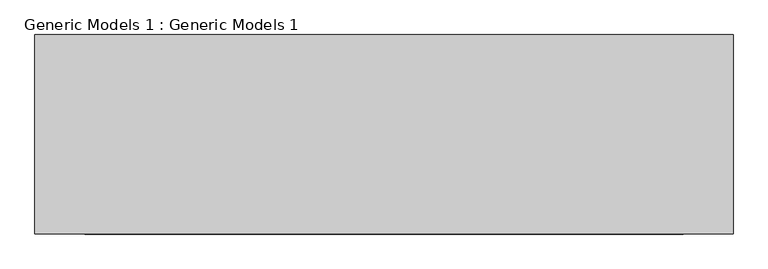
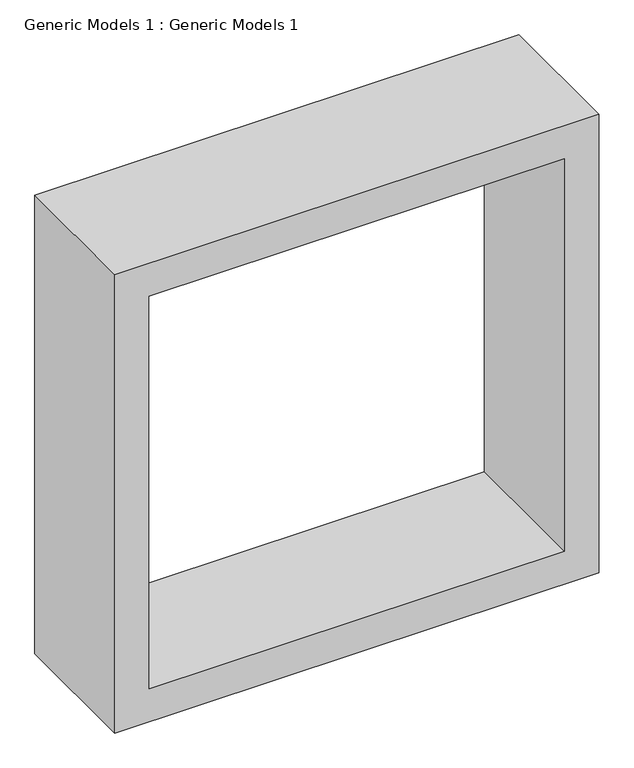
"""IFC4 building model written with IfcOpenShell, lengths in millimetres: proxy geometry, Generic Models 1 : Generic Models 1."""

from ifc_helpers import new_model, si_unit, frame, origin, place, context, project, spatial, polyline, outline, extrude, source, transform, mapped, element, save


def generic_models_1_generic_models_1_e3b611d6(model_context):
    return source(origin(), model_context, "Body", "SweptSolid", [
        extrude(outline(polyline([(6705.6, -8954.4294011), (6705.6, -11088.0294011), (4572.0, -11088.0294011), (4572.0, -8954.4294011), (6705.6, -8954.4294011)]), holes=[polyline([(6553.2, -9106.8294011), (4724.4, -9106.8294011), (4724.4, -10935.6294011), (6553.2, -10935.6294011), (6553.2, -9106.8294011)])]), frame((0.0, -2991.5111529, 0.0), z_axis=(0.0, 1.0, 0.0), x_axis=(0.0, 0.0, 1.0)), (0.0, 0.0, 1.0), 609.6),
    ])


if __name__ == "__main__":
    model = new_model("IFC4")
    model_context = context("Model", 3, world=origin())
    ifc_project = project(units=[si_unit("LENGTHUNIT", "METRE", prefix="MILLI")], contexts=[model_context])
    site = spatial("IfcSite", under=ifc_project)
    building = spatial("IfcBuilding", under=site)
    placement = place(None, origin())
    generic_models_1_generic_models_1_shape = generic_models_1_generic_models_1_e3b611d6(model_context)
    element("IfcBuildingElementProxy", 1, Name="Generic Models 1 : Generic Models 1", ObjectType="Generic Models 1 : Generic Models 1", at=placement, inside=building, context=model_context, shape_type="MappedRepresentation", body=[
        mapped(generic_models_1_generic_models_1_shape, transform((0.0, 0.0, 0.0), x_axis=(1.0, 0.0, 0.0), y_axis=(0.0, 1.0, 0.0), z_axis=(0.0, 0.0, 1.0))),
    ])
    save(model, "model.ifc")

# Revit data of these elements
# Element 1 (IfcBuildingElementProxy, "Generic Models 1 : Generic Models 1")
#   Materials on its faces: "Gypsum Wall Board"
# Materials
#   "Gypsum Wall Board": class "Generic", colour RGB 127 127 127, transparency 0, Description = "Gypsum Wall Board", Cost = 0
